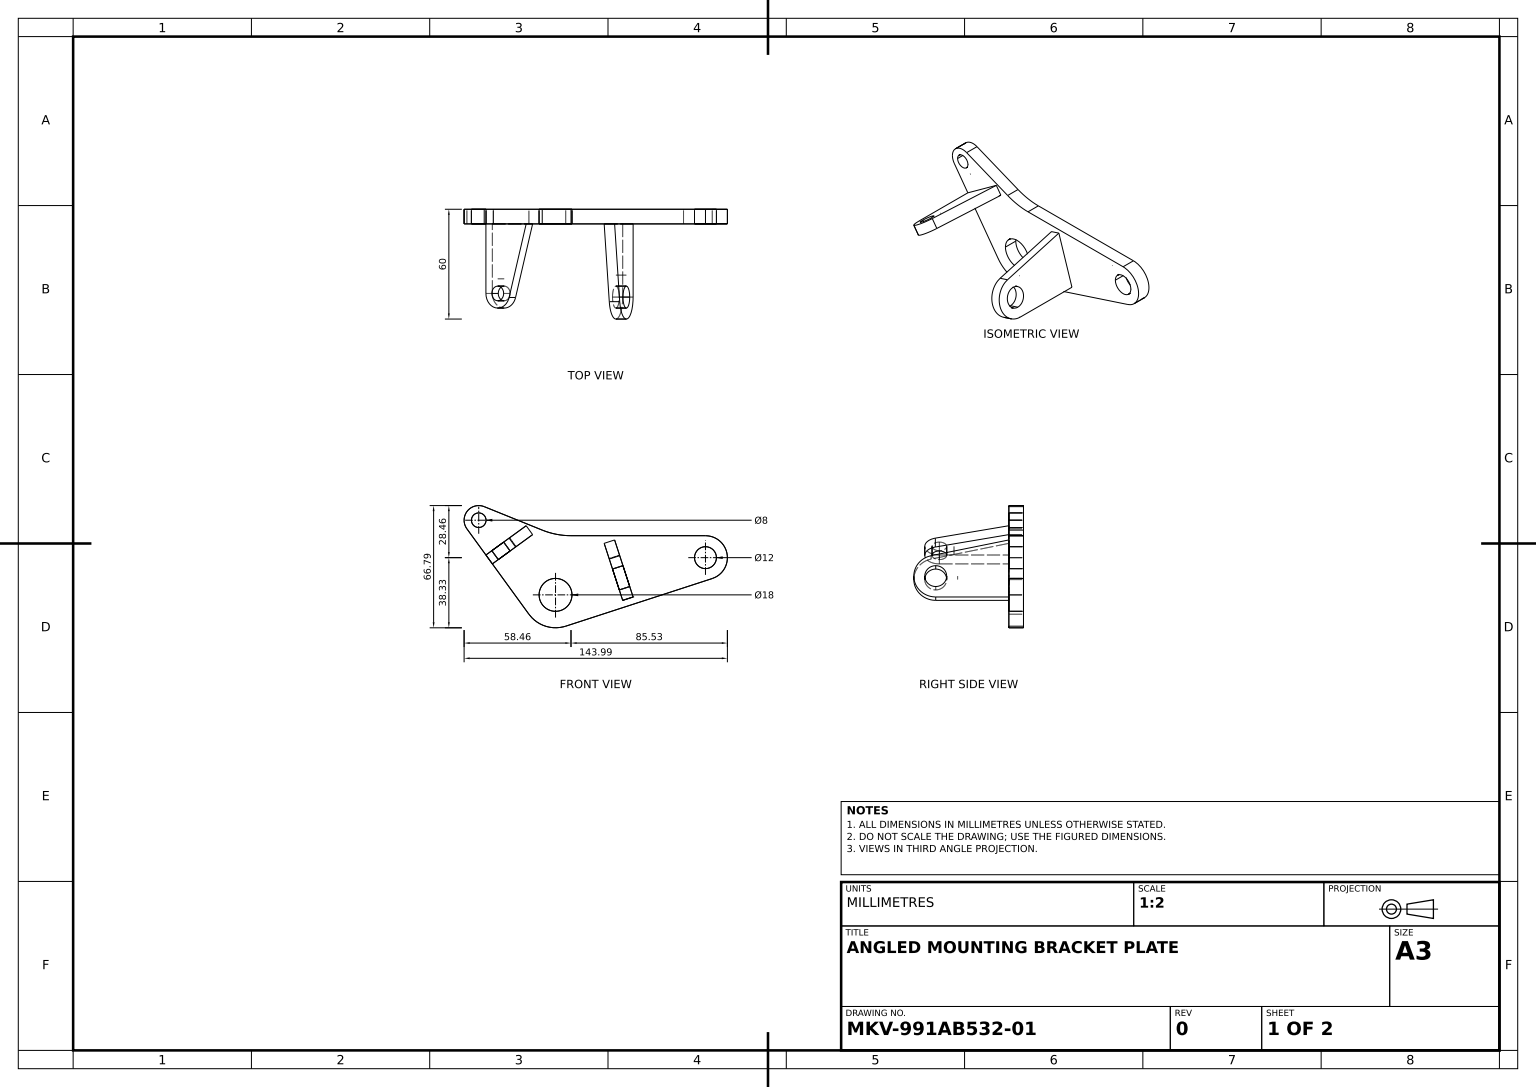
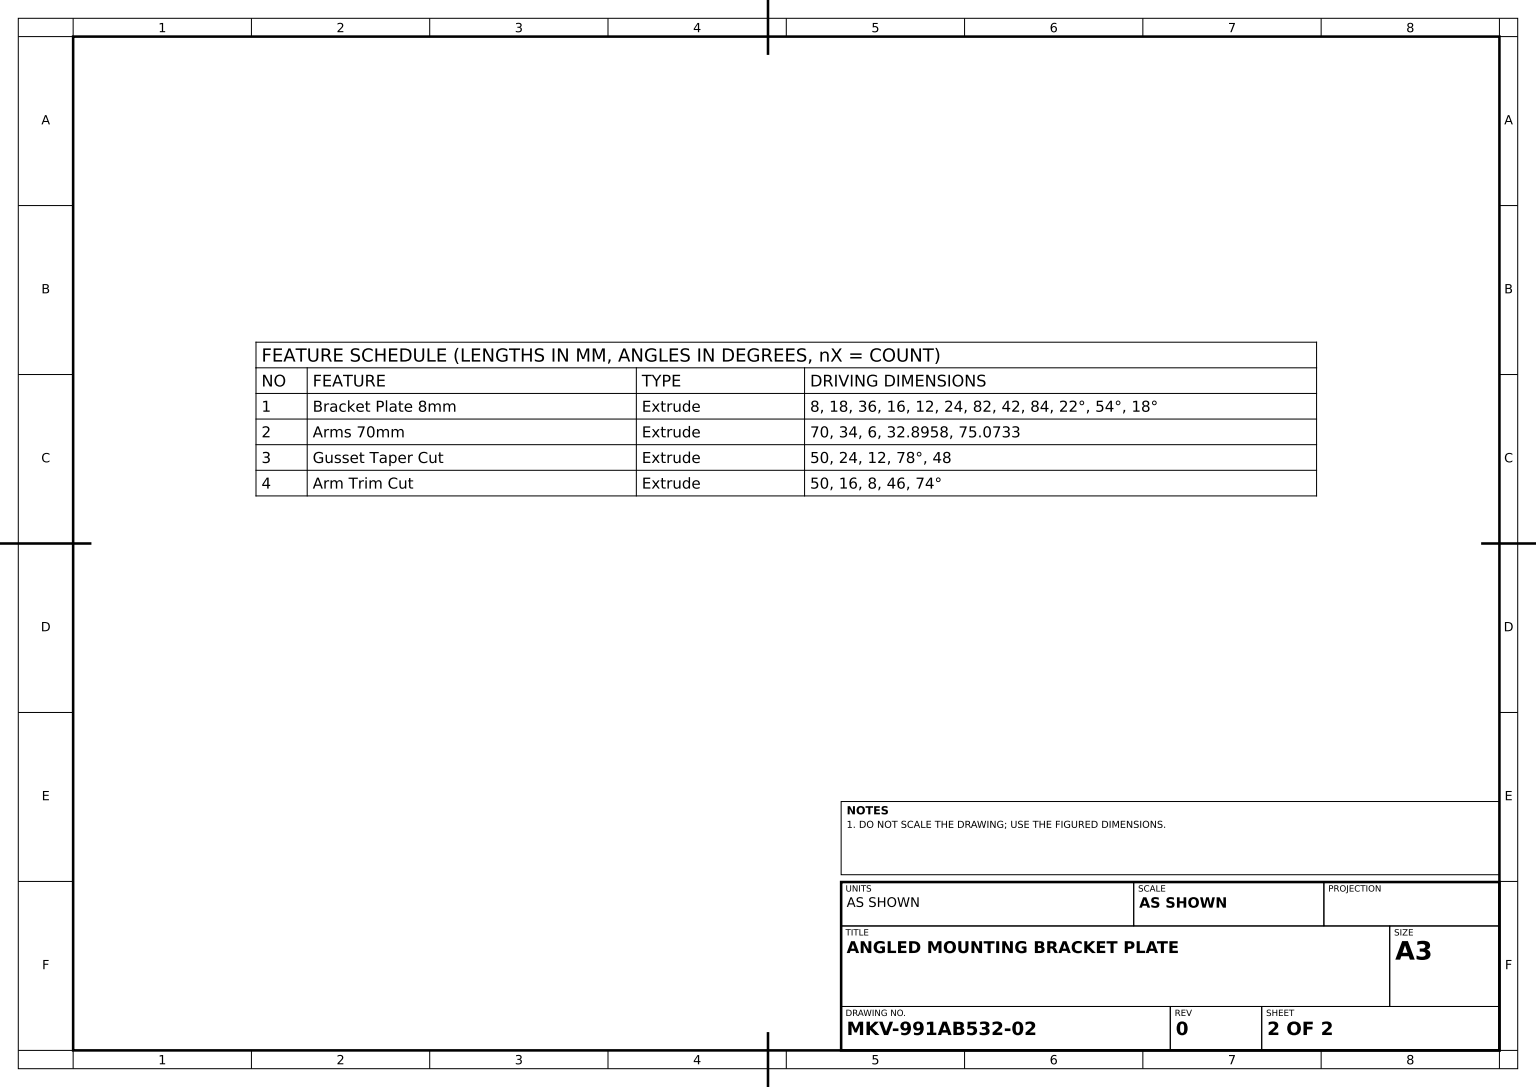
from build123d import *

# Parameters (mm, degrees)
BRACKET_PLATE_PROFILE_R    = 9
BRACKET_PLATE_PROFILE_R_2  = 4
BRACKET_PLATE_PROFILE_R_3  = 6
BRACKET_PLATE_8MM_DEPTH    = 8
ARMS_70MM_DEPTH            = 70
GUSSET_TAPER_CUT_PROFILE_R = 6
GUSSET_TAPER_CUT_DEPTH     = 50
ARM_TRIM_CUT_PROFILE_R     = 4
ARM_TRIM_CUT_DEPTH         = 50


with BuildPart() as part:
    # Bracket Plate Profile → Bracket Plate 8mm (new body)
    with BuildSketch(Plane.XY):
        with BuildLine():
            Line((-48.472135955, 36.092742474), (-14.562305899, -10.580134541))
            ThreePointArc((-14.562305899, -10.580134541), (-5.562305899, -17.119017293), (5.562305899, -17.119017293))
            Line((5.562305899, -17.119017293), (85.708203932, 8.92196355))
            ThreePointArc((85.708203932, 8.92196355), (93.852260087, 22.211855326), (82, 32.334641746))
            Line((82, 32.334641746), (8.459892396, 32.334641746))
            ThreePointArc((8.459892396, 32.334641746), (0.445914591, 33.106300041), (-7.273584527, 35.392919854))
            Line((-7.273584527, 35.392919854), (-39.003147253, 48.212495329))
            ThreePointArc((-39.003147253, 48.212495329), (-48.304086029, 45.720316295), (-48.472135955, 36.092742474))
        make_face()
        Circle(BRACKET_PLATE_PROFILE_R, mode=Mode.SUBTRACT)
        with Locations((-42, 40.795024493)):
            Circle(BRACKET_PLATE_PROFILE_R_2, mode=Mode.SUBTRACT)
        with Locations((82, 20.334641746)):
            Circle(BRACKET_PLATE_PROFILE_R_3, mode=Mode.SUBTRACT)
    extrude(amount=BRACKET_PLATE_8MM_DEPTH)

    # Arm Sections 34x6 → Arms 70mm (add)
    with BuildSketch(Plane.XY.offset(8)):
        Polygon((37.898227453, -6.612439485), (43.604566551, -4.758337518), (32.307498994, 30.01046132), (26.601159896, 28.156359354), align=None)
        Polygon((-38.07371599, 21.780545234), (-34.547004477, 16.926443267), (-12.049603456, 33.271761878), (-15.57631497, 38.125863845), align=None)
    extrude(amount=ARMS_70MM_DEPTH)

    # Gusset Taper Cut Profile → Gusset Taper Cut (cut)
    with BuildSketch(Plane(origin=(38.042260652, 12.360679775, 0), x_dir=(0, 0, -1), z_dir=(0.9510565162951532, 0.30901699437494873, 0))):
        with BuildLine():
            Line((-50.49494029, 9.525500165), (-8, 18.558078561))
            Line((-8, 18.558078561), (-78, 18.558078561))
            Line((-78, 18.558078561), (-78, -18))
            Line((-78, -18), (-8, -18))
            Line((-8, -18), (-8, -14.212271044))
            Line((-8, -14.212271044), (-48, -14.212271044))
            ThreePointArc((-48, -14.212271044), (-59.934262744, -3.466612603), (-50.49494029, 9.525500165))
        make_face()
        with Locations(Location((-48, -2.212271044, 0), (0, 0, 90))):
            Circle(GUSSET_TAPER_CUT_PROFILE_R)
    extrude(amount=-GUSSET_TAPER_CUT_DEPTH, mode=Mode.SUBTRACT)

    # Arm Trim Cut Profile → Arm Trim Cut (cut)
    with BuildSketch(Plane(origin=(-23.511410092, 32.360679775, 0), x_dir=(0.8090169943749487, 0.5877852522924716, 0), z_dir=(-0.5877852522924715, 0.8090169943749486, 0))):
        with Locations(Location((-10, -46, 0), (0, 0, 180))):
            Circle(ARM_TRIM_CUT_PROFILE_R)
        with BuildLine():
            Line((9.808316978, -8), (9.218720146, -8))
            Line((9.218720146, -8), (-2.309906432, -48.205098847))
            ThreePointArc((-2.309906432, -48.205098847), (-11.113384808, -53.92214455), (-18, -46))
            Line((-18, -46), (-18, -78))
            Line((-18, -78), (9.808316978, -78))
            Line((9.808316978, -78), (9.808316978, -8))
        make_face()
    extrude(amount=-ARM_TRIM_CUT_DEPTH, mode=Mode.SUBTRACT)


solid = part.part
